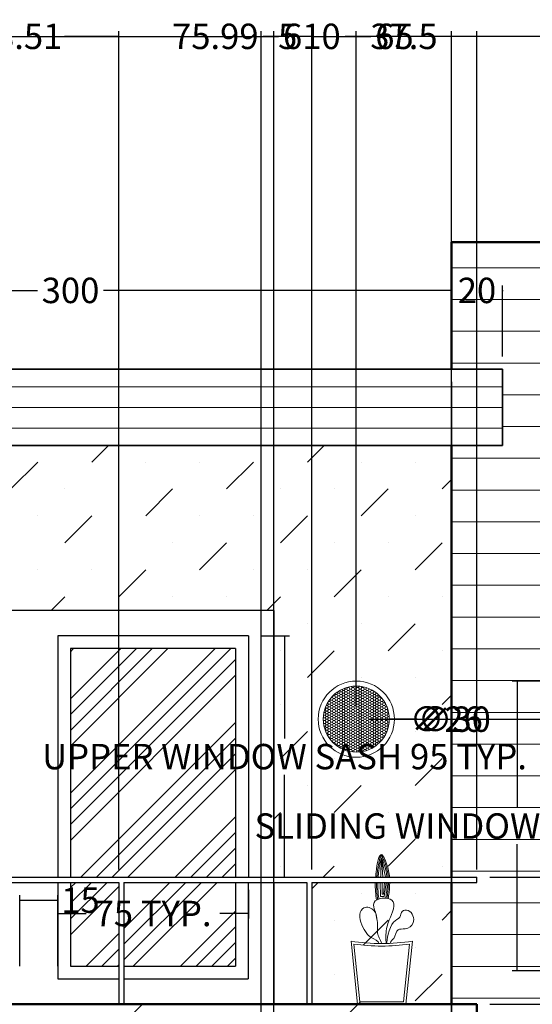
# Model space of a CAD drawing. Units: millimetres. Extents: x 301 to 1039, y -12 to 673.
# Tile 4 of 6: x 534 to 736, y 285 to 673. Entities that reach past the tile are written whole.
import ezdxf

# ---------------------------------------------------------------- set-up
doc = ezdxf.new("R2010")
doc.units = ezdxf.units.MM
doc.header["$MEASUREMENT"] = 0
for name, color, linetype, lineweight in [('A-ANNO-DIMS', 2, 'Continuous', 18), ('A-EQPM', 8, 'Continuous', 18), ('A-FLOR-HRAL', 6, 'Continuous', 25), ('A-GLAZ', 4, 'Continuous', 25), ('A-GLAZ-PATT', 8, 'Continuous', 13), ('A-ROOF', 1, 'Continuous', 35), ('A-WALL', 7, 'Continuous', 50), ('A-WALL-PATT', 9, 'Continuous', 13), ('L-PLNT', 3, 'Continuous', 18)]:
    doc.layers.add(name, color=color, linetype=linetype, lineweight=lineweight)
doc.styles.get("Standard").update_dxf_attribs({"font": 'arial.ttf'})
doc.dimstyles.get("Standard").update_dxf_attribs({"dimtxt": 10, "dimasz": 0.18, "dimexe": 2, "dimexo": 5, "dimgap": 2, "dimtad": 0, "dimtih": 1, "dimtoh": 1, "dimdec": 0, "dimzin": 0, "dimdsep": 46, "dimtxsty": 'Standard', "dimcen": 0.09, "dimadec": 0, "dimazin": 0, "dimtfac": 1, "dimtdec": 0, "dimtofl": 0, "dimtmove": 0, "dimatfit": 3, "dimfxl": 1, "dimtolj": 1, "dimtzin": 0, "dimarcsym": 0})

# ---------------------------------------------------------------- blocks, each defined once
blk = doc.blocks.new('WIN-SASH-UPPER')
for p, q in [((623.79, 430.09), (548.79, 430.09)), ((548.79, 430.09), (548.79, 400.52)), ((623.79, 430.09), (623.79, 400.52)), ((618.79, 425.09), (553.79, 425.09)), ((553.79, 425.09), (553.79, 400.52)), ((618.79, 425.09), (618.79, 400.52)), ((548.79, 400.52), (548.79, 335.09)), ((553.79, 400.52), (553.79, 335.09)), ((618.79, 400.52), (618.79, 335.09)), ((623.79, 400.52), (623.79, 335.09))]:
    blk.add_line(p, q)
blk = doc.blocks.new('*D12')
at = {"layer": 'A-ANNO-DIMS', "color": 0, "lineweight": -2, "transparency": 16777216}
for p, q in [((628.79, 430.09), (640.04, 430.09)), ((638.04, 429.91), (638.04, 389.76)), ((638.04, 335.27), (638.04, 375.41)), ((628.79, 335.09), (640.04, 335.09))]:
    blk.add_line(p, q, dxfattribs=at)
at = {"layer": 'A-ANNO-DIMS', "color": 0, "transparency": 16777216}
for points in [[(638.01, 429.91), (638.07, 429.91), (638.04, 430.09)], [(638.01, 335.27), (638.07, 335.27), (638.04, 335.09)]]:
    blk.add_solid(points, dxfattribs=at)
at = {"layer": 'Defpoints', "color": 0, "transparency": 16777216}
for p in [(623.79, 430.09), (638.04, 430.09), (623.79, 335.09)]:
    blk.add_point(p, dxfattribs=at)
at = {"layer": 'A-ANNO-DIMS', "color": 0, "transparency": 16777216, "insert": (638.04, 382.59), "char_height": 10, "attachment_point": 5}
blk.add_mtext('\\A1;UPPER WINDOW SASH 95 TYP.', dxfattribs=at)
blk = doc.blocks.new('*D13')
at = {"layer": 'A-ANNO-DIMS', "color": 0, "lineweight": -2, "transparency": 16777216}
for p, q in [((548.79, 330.09), (548.79, 318.84)), ((623.79, 330.09), (623.79, 318.84)), ((548.97, 320.84), (559.99, 320.84)), ((623.61, 320.84), (612.59, 320.84))]:
    blk.add_line(p, q, dxfattribs=at)
at = {"layer": 'A-ANNO-DIMS', "color": 0, "transparency": 16777216}
for points in [[(548.97, 320.87), (548.97, 320.81), (548.79, 320.84)], [(623.61, 320.87), (623.61, 320.81), (623.79, 320.84)]]:
    blk.add_solid(points, dxfattribs=at)
at = {"layer": 'Defpoints', "color": 0, "transparency": 16777216}
for p in [(548.79, 335.09), (623.79, 335.09), (623.79, 320.84)]:
    blk.add_point(p, dxfattribs=at)
at = {"layer": 'A-ANNO-DIMS', "color": 0, "transparency": 16777216, "insert": (586.29, 320.84), "char_height": 10, "attachment_point": 5}
blk.add_mtext('\\A1;75 TYP.', dxfattribs=at)
blk = doc.blocks.new('*D16')
at = {"layer": 'A-ANNO-DIMS', "color": 0, "lineweight": -2, "transparency": 16777216}
for p, q in [((741.69, 412.26), (727.59, 412.26)), ((729.59, 412.08), (729.59, 362.44)), ((729.59, 298.44), (729.59, 348.09)), ((741.69, 298.26), (727.59, 298.26))]:
    blk.add_line(p, q, dxfattribs=at)
at = {"layer": 'A-ANNO-DIMS', "color": 0, "transparency": 16777216}
for points in [[(729.56, 412.08), (729.62, 412.08), (729.59, 412.26)], [(729.56, 298.44), (729.62, 298.44), (729.59, 298.26)]]:
    blk.add_solid(points, dxfattribs=at)
at = {"layer": 'Defpoints', "color": 0, "transparency": 16777216}
for p in [(729.59, 412.26), (746.69, 412.26), (746.69, 298.26)]:
    blk.add_point(p, dxfattribs=at)
at = {"layer": 'A-ANNO-DIMS', "color": 0, "transparency": 16777216, "insert": (729.59, 355.26), "char_height": 10, "attachment_point": 5}
blk.add_mtext('\\A1;SLIDING WINDOW SASH 114 TYP.', dxfattribs=at)
blk = doc.blocks.new('*D20')
at = {"layer": 'A-ANNO-DIMS', "color": 0, "lineweight": -2, "transparency": 16777216}
for p, q in [((343.79, 30.09), (343.79, 668.09)), ((953.79, 30.09), (953.79, 668.09)), ((343.97, 666.09), (635.73, 666.09)), ((953.61, 666.09), (661.85, 666.09))]:
    blk.add_line(p, q, dxfattribs=at)
at = {"layer": 'A-ANNO-DIMS', "color": 0, "transparency": 16777216}
for points in [[(343.97, 666.12), (343.97, 666.06), (343.79, 666.09)], [(953.61, 666.12), (953.61, 666.06), (953.79, 666.09)]]:
    blk.add_solid(points, dxfattribs=at)
at = {"layer": 'Defpoints', "color": 0, "transparency": 16777216}
for p in [(953.79, 666.09), (343.79, 25.09), (953.79, 25.09)]:
    blk.add_point(p, dxfattribs=at)
at = {"layer": 'A-ANNO-DIMS', "color": 0, "transparency": 16777216, "insert": (648.79, 666.09), "char_height": 10, "attachment_point": 5}
blk.add_mtext('\\A1;610', dxfattribs=at)
blk = doc.blocks.new('*D26')
at = {"layer": 'A-ANNO-DIMS', "color": 0, "lineweight": -2, "transparency": 16777216}
for p, q in [((703.79, 530.09), (703.79, -7.91)), ((613.79, 30.09), (613.79, -7.91)), ((613.97, -5.91), (649.64, -5.91)), ((703.61, -5.91), (667.93, -5.91))]:
    blk.add_line(p, q, dxfattribs=at)
at = {"layer": 'A-ANNO-DIMS', "color": 0, "transparency": 16777216}
for points in [[(613.97, -5.88), (613.97, -5.94), (613.79, -5.91)], [(703.61, -5.88), (703.61, -5.94), (703.79, -5.91)]]:
    blk.add_solid(points, dxfattribs=at)
at = {"layer": 'Defpoints', "color": 0, "transparency": 16777216}
for p in [(703.79, 535.09), (613.79, 35.09), (703.79, -5.91)]:
    blk.add_point(p, dxfattribs=at)
at = {"layer": 'A-ANNO-DIMS', "color": 0, "transparency": 16777216, "insert": (658.79, -5.91), "char_height": 10, "attachment_point": 5}
blk.add_mtext('\\A1;90', dxfattribs=at)
blk = doc.blocks.new('*D27')
at = {"layer": 'A-ANNO-DIMS', "color": 0, "lineweight": -2, "transparency": 16777216}
for p, q in [((703.79, 530.09), (703.79, -7.91)), ((728.79, 155.09), (728.79, -7.91)), ((703.97, -5.91), (707, -5.91)), ((728.61, -5.91), (725.57, -5.91))]:
    blk.add_line(p, q, dxfattribs=at)
at = {"layer": 'A-ANNO-DIMS', "color": 0, "transparency": 16777216}
for points in [[(703.97, -5.88), (703.97, -5.94), (703.79, -5.91)], [(728.61, -5.88), (728.61, -5.94), (728.79, -5.91)]]:
    blk.add_solid(points, dxfattribs=at)
at = {"layer": 'Defpoints', "color": 0, "transparency": 16777216}
for p in [(703.79, 535.09), (728.79, 160.09), (728.79, -5.91)]:
    blk.add_point(p, dxfattribs=at)
at = {"layer": 'A-ANNO-DIMS', "color": 0, "transparency": 16777216, "insert": (716.29, -5.91), "char_height": 10, "attachment_point": 5}
blk.add_mtext('\\A1;25', dxfattribs=at)
blk = doc.blocks.new('*D44')
at = {"layer": 'A-ANNO-DIMS', "color": 0, "lineweight": -2, "transparency": 16777216}
for p, q in [((403.79, 540.09), (403.79, 568.09)), ((403.97, 566.09), (540.76, 566.09)), ((703.61, 566.09), (566.82, 566.09)), ((703.79, 540.09), (703.79, 568.09))]:
    blk.add_line(p, q, dxfattribs=at)
at = {"layer": 'A-ANNO-DIMS', "color": 0, "transparency": 16777216}
for points in [[(403.97, 566.12), (403.97, 566.06), (403.79, 566.09)], [(703.61, 566.12), (703.61, 566.06), (703.79, 566.09)]]:
    blk.add_solid(points, dxfattribs=at)
at = {"layer": 'Defpoints', "color": 0, "transparency": 16777216}
for p in [(703.79, 566.09), (403.79, 535.09), (703.79, 535.09)]:
    blk.add_point(p, dxfattribs=at)
at = {"layer": 'A-ANNO-DIMS', "color": 0, "transparency": 16777216, "insert": (553.79, 566.09), "char_height": 10, "attachment_point": 5}
blk.add_mtext('\\A1;300', dxfattribs=at)
blk = doc.blocks.new('*D45')
at = {"layer": 'A-ANNO-DIMS', "color": 0, "lineweight": -2, "transparency": 16777216}
for p, q in [((703.608413, 566.088152), (703.428413, 566.088152)), ((703.788413, 540.088152), (703.788413, 568.088152)), ((723.788413, 540.088152), (723.788413, 568.088152)), ((723.968413, 566.088152), (724.148413, 566.088152))]:
    blk.add_line(p, q, dxfattribs=at)
at = {"layer": 'A-ANNO-DIMS', "color": 0, "transparency": 16777216}
for points in [[(703.608413, 566.118152), (703.608413, 566.058152), (703.788413, 566.088152)], [(723.968413, 566.118152), (723.968413, 566.058152), (723.788413, 566.088152)]]:
    blk.add_solid(points, dxfattribs=at)
at = {"layer": 'Defpoints', "color": 0, "transparency": 16777216}
for p in [(723.788413, 566.088152), (703.788413, 535.088152), (723.788413, 535.088152)]:
    blk.add_point(p, dxfattribs=at)
at = {"layer": 'A-ANNO-DIMS', "color": 0, "transparency": 16777216, "insert": (713.788413, 566.088152), "char_height": 10, "attachment_point": 5}
blk.add_mtext('\\A1;20', dxfattribs=at)
blk = doc.blocks.new('*D52')
at = {"layer": 'A-ANNO-DIMS', "color": 0, "lineweight": -2, "transparency": 16777216}
for p, q in [((666.29, 402.33), (666.29, 668.09)), ((703.79, 265.09), (703.79, 668.09)), ((666.47, 666.09), (670.02, 666.09)), ((703.61, 666.09), (700.06, 666.09))]:
    blk.add_line(p, q, dxfattribs=at)
at = {"layer": 'A-ANNO-DIMS', "color": 0, "transparency": 16777216}
for points in [[(666.47, 666.12), (666.47, 666.06), (666.29, 666.09)], [(703.61, 666.12), (703.61, 666.06), (703.79, 666.09)]]:
    blk.add_solid(points, dxfattribs=at)
at = {"layer": 'Defpoints', "color": 0, "transparency": 16777216}
for p in [(703.79, 666.09), (666.29, 397.33), (703.79, 260.09)]:
    blk.add_point(p, dxfattribs=at)
at = {"layer": 'A-ANNO-DIMS', "color": 0, "transparency": 16777216, "insert": (685.04, 666.09), "char_height": 10, "attachment_point": 5}
blk.add_mtext('\\A1;37.5', dxfattribs=at)
blk = doc.blocks.new('*D56')
at = {"layer": 'A-ANNO-DIMS', "color": 0, "lineweight": -2, "transparency": 16777216}
for p, q in [((718.79, 335.09), (986.79, 335.09)), ((984.79, 334.91), (984.79, 317.19)), ((984.79, 285.27), (984.79, 302.98)), ((718.79, 285.09), (986.79, 285.09))]:
    blk.add_line(p, q, dxfattribs=at)
at = {"layer": 'A-ANNO-DIMS', "color": 0, "transparency": 16777216}
for points in [[(984.76, 334.91), (984.82, 334.91), (984.79, 335.09)], [(984.76, 285.27), (984.82, 285.27), (984.79, 285.09)]]:
    blk.add_solid(points, dxfattribs=at)
at = {"layer": 'Defpoints', "color": 0, "transparency": 16777216}
for p in [(713.79, 335.09), (984.79, 335.09), (713.79, 285.09)]:
    blk.add_point(p, dxfattribs=at)
at = {"layer": 'A-ANNO-DIMS', "color": 0, "transparency": 16777216, "insert": (984.79, 310.09), "char_height": 10, "attachment_point": 5}
blk.add_mtext('\\A1;50', dxfattribs=at)
blk = doc.blocks.new('*D57')
at = {"layer": 'A-ANNO-DIMS', "color": 0, "lineweight": -2, "transparency": 16777216}
for p, q in [((671.29, 397.33), (986.79, 397.33)), ((984.79, 397.15), (984.79, 373.32)), ((984.79, 335.27), (984.79, 359.11)), ((718.79, 335.09), (986.79, 335.09))]:
    blk.add_line(p, q, dxfattribs=at)
at = {"layer": 'A-ANNO-DIMS', "color": 0, "transparency": 16777216}
for points in [[(984.76, 397.15), (984.82, 397.15), (984.79, 397.33)], [(984.76, 335.27), (984.82, 335.27), (984.79, 335.09)]]:
    blk.add_solid(points, dxfattribs=at)
at = {"layer": 'Defpoints', "color": 0, "transparency": 16777216}
for p in [(666.29, 397.33), (984.79, 397.33), (713.79, 335.09)]:
    blk.add_point(p, dxfattribs=at)
at = {"layer": 'A-ANNO-DIMS', "color": 0, "transparency": 16777216, "insert": (984.79, 366.21), "char_height": 10, "attachment_point": 5}
blk.add_mtext('\\A1;62.25', dxfattribs=at)
blk = doc.blocks.new('*D60')
at = {"layer": 'A-ANNO-DIMS', "color": 0, "lineweight": -2, "transparency": 16777216}
for p, q in [((494.29, 338.09), (494.29, 668.09)), ((572.8, 338.09), (572.8, 668.09)), ((494.47, 666.09), (515.68, 666.09)), ((572.62, 666.09), (551.41, 666.09))]:
    blk.add_line(p, q, dxfattribs=at)
at = {"layer": 'A-ANNO-DIMS', "color": 0, "transparency": 16777216}
for points in [[(494.47, 666.12), (494.47, 666.06), (494.29, 666.09)], [(572.62, 666.12), (572.62, 666.06), (572.8, 666.09)]]:
    blk.add_solid(points, dxfattribs=at)
at = {"layer": 'Defpoints', "color": 0, "transparency": 16777216}
for p in [(572.8, 666.09), (494.29, 333.09), (572.8, 333.09)]:
    blk.add_point(p, dxfattribs=at)
at = {"layer": 'A-ANNO-DIMS', "color": 0, "transparency": 16777216, "insert": (533.54, 666.09), "char_height": 10, "attachment_point": 5}
blk.add_mtext('\\A1;78.51', dxfattribs=at)
blk = doc.blocks.new('*D61')
at = {"layer": 'A-ANNO-DIMS', "color": 0, "lineweight": -2, "transparency": 16777216}
for p, q in [((572.8, 338.09), (572.8, 668.09)), ((648.79, 338.09), (648.79, 668.09)), ((572.98, 666.09), (591.95, 666.09)), ((648.61, 666.09), (629.64, 666.09))]:
    blk.add_line(p, q, dxfattribs=at)
at = {"layer": 'A-ANNO-DIMS', "color": 0, "transparency": 16777216}
for points in [[(572.98, 666.12), (572.98, 666.06), (572.8, 666.09)], [(648.61, 666.12), (648.61, 666.06), (648.79, 666.09)]]:
    blk.add_solid(points, dxfattribs=at)
at = {"layer": 'Defpoints', "color": 0, "transparency": 16777216}
for p in [(648.79, 666.09), (572.8, 333.09), (648.79, 333.09)]:
    blk.add_point(p, dxfattribs=at)
at = {"layer": 'A-ANNO-DIMS', "color": 0, "transparency": 16777216, "insert": (610.79, 666.09), "char_height": 10, "attachment_point": 5}
blk.add_mtext('\\A1;75.99', dxfattribs=at)
blk = doc.blocks.new('*D62')
at = {"layer": 'A-ANNO-DIMS', "color": 0, "lineweight": -2, "transparency": 16777216}
for p, q in [((648.79, 338.09), (648.79, 668.09)), ((713.79, 338.09), (713.79, 668.09)), ((648.97, 666.09), (672.06, 666.09)), ((713.61, 666.09), (690.52, 666.09))]:
    blk.add_line(p, q, dxfattribs=at)
at = {"layer": 'A-ANNO-DIMS', "color": 0, "transparency": 16777216}
for points in [[(648.97, 666.12), (648.97, 666.06), (648.79, 666.09)], [(713.61, 666.12), (713.61, 666.06), (713.79, 666.09)]]:
    blk.add_solid(points, dxfattribs=at)
at = {"layer": 'Defpoints', "color": 0, "transparency": 16777216}
for p in [(713.79, 666.09), (648.79, 333.09), (713.79, 333.09)]:
    blk.add_point(p, dxfattribs=at)
at = {"layer": 'A-ANNO-DIMS', "color": 0, "transparency": 16777216, "insert": (681.29, 666.09), "char_height": 10, "attachment_point": 5}
blk.add_mtext('\\A1;65', dxfattribs=at)
blk = doc.blocks.new('*D63')
at = {"layer": 'A-ANNO-DIMS', "color": 0, "lineweight": -2, "transparency": 16777216}
for p, q in [((533.79, 300.09), (533.79, 328.09)), ((533.97, 326.09), (548.61, 326.09)), ((548.79, 300.09), (548.79, 328.09)), ((548.79, 326.09), (548.97, 326.09))]:
    blk.add_line(p, q, dxfattribs=at)
at = {"layer": 'A-ANNO-DIMS', "color": 0, "transparency": 16777216}
for points in [[(533.97, 326.12), (533.97, 326.06), (533.79, 326.09)], [(548.61, 326.12), (548.61, 326.06), (548.79, 326.09)]]:
    blk.add_solid(points, dxfattribs=at)
at = {"layer": 'Defpoints', "color": 0, "transparency": 16777216}
for p in [(548.79, 326.09), (533.79, 295.09), (548.79, 295.09)]:
    blk.add_point(p, dxfattribs=at)
at = {"layer": 'A-ANNO-DIMS', "color": 0, "transparency": 16777216, "insert": (557.7, 326.09), "char_height": 10, "attachment_point": 5}
blk.add_mtext('\\A1;15', dxfattribs=at)
blk = doc.blocks.new('*D72')
at = {"layer": 'A-ANNO-DIMS', "color": 0, "lineweight": -2, "transparency": 16777216}
for p, q in [((628.79, 190.09), (628.79, 668.09)), ((633.79, 185.09), (633.79, 668.09)), ((628.97, 666.09), (633.61, 666.09)), ((633.79, 666.09), (633.97, 666.09))]:
    blk.add_line(p, q, dxfattribs=at)
at = {"layer": 'A-ANNO-DIMS', "color": 0, "transparency": 16777216}
for points in [[(628.97, 666.12), (628.97, 666.06), (628.79, 666.09)], [(633.61, 666.12), (633.61, 666.06), (633.79, 666.09)]]:
    blk.add_solid(points, dxfattribs=at)
at = {"layer": 'Defpoints', "color": 0, "transparency": 16777216}
for p in [(633.79, 666.09), (628.79, 185.09), (633.79, 180.09)]:
    blk.add_point(p, dxfattribs=at)
at = {"layer": 'A-ANNO-DIMS', "color": 0, "transparency": 16777216, "insert": (639.28, 666.09), "char_height": 10, "attachment_point": 5}
blk.add_mtext('\\A1;5', dxfattribs=at)
blk = doc.blocks.new('*D79')
at = {"layer": 'A-ANNO-DIMS', "color": 0, "lineweight": -2, "transparency": 16777216}
for p, q in [((666.2, 397.33), (666.38, 397.33)), ((666.29, 397.24), (666.29, 397.42)), ((690.29, 397.33), (681.47, 397.33))]:
    blk.add_line(p, q, dxfattribs=at)
at = {"layer": 'A-ANNO-DIMS', "color": 0, "transparency": 16777216}
blk.add_solid([(681.47, 397.36), (681.47, 397.3), (681.29, 397.33)], dxfattribs=at)
at = {"layer": 'Defpoints', "color": 0, "transparency": 16777216}
for p in [(651.29, 397.34), (681.29, 397.33)]:
    blk.add_point(p, dxfattribs=at)
at = {"layer": 'A-ANNO-DIMS', "color": 0, "transparency": 16777216, "insert": (704.88, 397.33), "char_height": 10, "attachment_point": 5}
blk.add_mtext('\\A1;∅30', dxfattribs=at)
blk = doc.blocks.new('*D80')
at = {"layer": 'A-ANNO-DIMS', "color": 0, "lineweight": -2, "transparency": 16777216}
for p, q in [((666.2, 397.33), (666.38, 397.33)), ((666.29, 397.24), (666.29, 397.42)), ((687.09, 397.33), (679.47, 397.33))]:
    blk.add_line(p, q, dxfattribs=at)
at = {"layer": 'A-ANNO-DIMS', "color": 0, "transparency": 16777216}
blk.add_solid([(679.47, 397.36), (679.47, 397.3), (679.29, 397.33)], dxfattribs=at)
at = {"layer": 'Defpoints', "color": 0, "transparency": 16777216}
for p in [(653.29, 397.34), (679.29, 397.33)]:
    blk.add_point(p, dxfattribs=at)
at = {"layer": 'A-ANNO-DIMS', "color": 0, "transparency": 16777216, "insert": (701.69, 397.33), "char_height": 10, "attachment_point": 5}
blk.add_mtext('\\A1;∅26', dxfattribs=at)

msp = doc.modelspace()

# ---------------------------------------------------------------- hatches: boundary and pattern name
at = {"layer": 'A-EQPM'}
h = msp.add_hatch(dxfattribs=at)
h.set_pattern_fill('HONEY', color=256, scale=5)
h.paths.add_polyline_path([(653.292, 397.334, 1), (679.292, 397.334, 1)])
at = {"layer": 'A-GLAZ-PATT'}
h = msp.add_hatch(dxfattribs=at)
h.set_pattern_fill('ANSI34', color=256, scale=35)
h.paths.add_polyline_path([(528.788, 400.52), (528.788, 425.088), (463.788, 425.088), (463.788, 400.52), (463.788, 335.088), (528.788, 335.088)])
h.paths.add_polyline_path([(494.288, 333.088), (463.788, 333.088), (463.788, 300.088), (494.288, 300.088)])
h.paths.add_polyline_path([(528.788, 333.088), (496.288, 333.088), (496.288, 300.088), (528.788, 300.088)])
h.paths.add_polyline_path([(618.788, 400.52), (618.788, 425.088), (553.788, 425.088), (553.788, 400.52), (553.788, 335.088), (618.788, 335.088)])
h.paths.add_polyline_path([(618.788, 333.088), (574.798, 333.088), (574.798, 300.088), (618.788, 300.088)])
h.paths.add_polyline_path([(572.798, 333.088), (553.788, 333.088), (553.788, 300.088), (572.798, 300.088)])
h.paths.add_polyline_path([(501.288, 180.088), (433.788, 180.088), (433.788, 110.088), (501.288, 110.088)])
h.paths.add_polyline_path([(573.788, 180.088), (506.288, 180.088), (506.288, 110.088), (573.788, 110.088)])
h.paths.add_polyline_path([(573.788, 210.088), (506.288, 210.088), (506.288, 185.088), (573.788, 185.088)])
h.paths.add_polyline_path([(501.288, 210.088), (433.788, 210.088), (433.788, 185.088), (501.288, 185.088)])
h.paths.add_polyline_path([(797.687, 412.264), (746.687, 412.264), (746.687, 298.264), (797.687, 298.264)])
h.paths.add_polyline_path([(860.687, 412.264), (809.687, 412.264), (809.687, 298.264), (860.687, 298.264)])
at = {"layer": 'A-WALL-PATT'}
h = msp.add_hatch(dxfattribs=at)
h.set_pattern_fill('ANSI31', color=256, scale=100, angle=135)
h.paths.add_polyline_path([(903.788, 585.088), (703.788, 585.088), (703.788, 535.088), (723.788, 535.088), (723.788, 505.088), (703.788, 505.088), (703.788, 335.088), (713.788, 335.088), (713.788, 333.088), (703.788, 333.088), (703.788, 285.088), (713.788, 285.088), (713.788, 265.672), (903.788, 265.672)])
h.paths.add_polyline_path([(868.687, 420.264), (868.687, 290.264), (738.687, 290.264), (738.687, 420.264)], flags=16)
h.paths.add_polyline_path([(866.687, 418.264), (866.687, 292.264), (740.687, 292.264), (740.687, 418.264)], flags=0)
h.paths.add_polyline_path([(861.687, 413.264), (861.687, 297.264), (745.687, 297.264), (745.687, 413.264)], flags=0)
h.paths.add_polyline_path([(860.687, 412.264), (860.687, 298.264), (809.687, 298.264), (809.687, 412.264)], flags=0)
h.paths.add_polyline_path([(797.687, 412.264), (797.687, 298.264), (746.687, 298.264), (746.687, 412.264)], flags=0)
h = msp.add_hatch(dxfattribs=at)
h.set_pattern_fill('ANSI31', color=256, scale=65, angle=135)
h.paths.add_polyline_path([(723.788, 535.088), (703.788, 535.088), (403.788, 535.088), (393.788, 535.088), (393.788, 505.088), (403.788, 505.088), (703.788, 505.088), (723.788, 505.088)])
h = msp.add_hatch(dxfattribs=at)
h.set_pattern_fill('MUDST', color=256, scale=60, angle=45)
edge = h.paths.add_edge_path()
edge.add_line((703.788, 505.088), (403.788, 505.088))
edge.add_line((403.788, 505.088), (403.788, 335.088))
edge.add_line((403.788, 335.088), (448.788, 335.088))
edge.add_line((448.788, 335.088), (448.788, 400.52))
edge.add_line((448.788, 400.52), (448.788, 440.088))
edge.add_line((448.788, 440.088), (633.788, 440.088))
edge.add_line((633.788, 440.088), (633.788, 400.52))
edge.add_line((633.788, 400.52), (633.788, 335.088))
edge.add_line((633.788, 335.088), (673.88, 335.088))
edge.add_spline(control_points=[(673.88, 335.088), (673.929, 335.734), (674.283, 339.462), (675.587, 346.794), (678.602, 339.909), (679.226, 336.718), (679.369, 335.088)], knot_values=[26.7052686, 26.7052686, 26.7052686, 26.7052686, 28.3156814, 35.5227919, 39.6456178, 44.5318346, 44.5318346, 44.5318346, 44.5318346], degree=3, periodic=0)
edge.add_line((679.369, 335.088), (703.788, 335.088))
edge.add_line((703.788, 335.088), (703.788, 505.088))
h.paths.add_polyline_path([(681.292, 397.334, -1), (651.292, 397.334, -1)], flags=16)
h.paths.add_polyline_path([(679.292, 397.334, -1), (653.292, 397.334, -1)], flags=0)
h.paths.add_polyline_path([(448.788, 333.088), (403.788, 333.088), (403.788, 285.088), (448.788, 285.088)])
h.paths.add_polyline_path([(613.788, 260.088), (713.788, 260.088), (713.788, 285.088), (403.788, 285.088), (393.788, 285.088), (393.788, 35.088), (403.788, 35.088), (613.788, 35.088)])
h.paths.add_polyline_path([(578.788, 215.088), (578.788, 105.088), (428.788, 105.088), (428.788, 215.088)], flags=16)
h.paths.add_polyline_path([(501.288, 210.088), (501.288, 185.088), (433.788, 185.088), (433.788, 210.088)], flags=0)
h.paths.add_polyline_path([(501.288, 180.088), (501.288, 110.088), (433.788, 110.088), (433.788, 180.088)], flags=0)
h.paths.add_polyline_path([(506.288, 210.088), (573.788, 210.088), (573.788, 185.088), (506.288, 185.088)], flags=0)
h.paths.add_polyline_path([(506.288, 180.088), (573.788, 180.088), (573.788, 110.088), (506.288, 110.088)], flags=0)
edge = h.paths.add_edge_path()
edge.add_spline(control_points=[(675.148, 309.006), (675.282, 309.92), (671.965, 311.304), (670.019, 313.17), (668.379, 316.485), (667.076, 320.028), (669.149, 324.142), (672.687, 322.877), (673.644, 321.553), (673.786, 321.296)], knot_values=[12.4980994, 12.4980994, 12.4980994, 12.4980994, 15.7345293, 18.1242776, 22.0598536, 26.1694355, 29.2709867, 33.3603853, 34.273637, 34.273637, 34.273637, 34.273637], degree=3, periodic=0)
edge.add_spline(control_points=[(673.786, 321.296), (673.373, 322.666), (672.565, 324.662), (673.805, 325.84), (674.246, 326.099)], knot_values=[12.3304253, 12.3304253, 12.3304253, 12.3304253, 16.1943692, 17.6683934, 17.6683934, 17.6683934, 17.6683934], degree=3, periodic=0)
edge.add_spline(control_points=[(674.246, 326.099), (673.92, 328.298), (673.697, 330.39), (673.774, 333.088)], knot_values=[46.2924512, 46.2924512, 46.2924512, 46.2924512, 53.8278009, 53.8278009, 53.8278009, 53.8278009], degree=3, periodic=0)
edge.add_line((673.774, 333.088), (648.788, 333.088))
edge.add_line((648.788, 333.088), (648.788, 285.088))
edge.add_line((648.788, 285.088), (666.788, 285.088))
edge.add_line((666.788, 285.088), (664.215, 309.96))
edge.add_arc((676.288, 385.148), 76.15, 260.87778, 269.14183)
edge = h.paths.add_edge_path()
edge.add_line((703.788, 333.088), (679.453, 333.088))
edge.add_spline(control_points=[(679.453, 333.088), (679.452, 331.277), (679.21, 329.205), (678.936, 327.067), (678.889, 326.706)], knot_values=[17.8386285, 17.8386285, 17.8386285, 17.8386285, 23.5111371, 24.6594022, 24.6594022, 24.6594022, 24.6594022], degree=3, periodic=0)
edge.add_spline(control_points=[(678.889, 326.706), (678.729, 326.741), (678.565, 326.771), (678.396, 326.794)], knot_values=[21.2892091, 21.2892091, 21.2892091, 21.2892091, 21.7264211, 21.7264211, 21.7264211, 21.7264211], degree=3, periodic=0)
edge.add_spline(control_points=[(678.396, 326.794), (678.233, 326.816), (678.067, 326.832), (677.898, 326.842)], knot_values=[20.8675669, 20.8675669, 20.8675669, 20.8675669, 21.2892091, 21.2892091, 21.2892091, 21.2892091], degree=3, periodic=0)
edge.add_spline(control_points=[(677.898, 326.842), (676.995, 326.898), (676.024, 326.786), (675.195, 326.517)], knot_values=[18.611077, 18.611077, 18.611077, 18.611077, 20.8675669, 20.8675669, 20.8675669, 20.8675669], degree=3, periodic=0)
edge.add_spline(control_points=[(675.195, 326.517), (675.029, 326.464), (674.869, 326.404), (674.716, 326.337)], knot_values=[18.1593829, 18.1593829, 18.1593829, 18.1593829, 18.611077, 18.611077, 18.611077, 18.611077], degree=3, periodic=0)
edge.add_spline(control_points=[(674.716, 326.337), (674.55, 326.265), (674.392, 326.186), (674.246, 326.099)], knot_values=[17.6683934, 17.6683934, 17.6683934, 17.6683934, 18.1593829, 18.1593829, 18.1593829, 18.1593829], degree=3, periodic=0)
edge.add_spline(control_points=[(674.246, 326.099), (673.805, 325.84), (672.565, 324.662), (673.373, 322.666), (673.786, 321.296)], knot_values=[12.3304253, 12.3304253, 12.3304253, 12.3304253, 13.8044495, 17.6683934, 17.6683934, 17.6683934, 17.6683934], degree=3, periodic=0)
edge.add_spline(control_points=[(673.786, 321.296), (674.162, 320.613), (674.301, 319.823), (674.341, 318.987)], knot_values=[10.0649388, 10.0649388, 10.0649388, 10.0649388, 12.4980994, 12.4980994, 12.4980994, 12.4980994], degree=3, periodic=0)
edge.add_spline(control_points=[(674.341, 318.987), (674.206, 319.737), (674.024, 320.504), (673.786, 321.296)], knot_values=[10.094462, 10.094462, 10.094462, 10.094462, 12.3304253, 12.3304253, 12.3304253, 12.3304253], degree=3, periodic=0)
edge.add_spline(control_points=[(673.786, 321.296), (673.644, 321.553), (672.687, 322.877), (669.149, 324.142), (667.076, 320.028), (668.379, 316.485), (670.019, 313.17), (671.965, 311.304), (675.282, 309.92), (675.148, 309.006)], knot_values=[12.4980994, 12.4980994, 12.4980994, 12.4980994, 13.4113511, 17.5007497, 20.6023009, 24.7118828, 28.6474588, 31.0372071, 34.273637, 34.273637, 34.273637, 34.273637], degree=3, periodic=0)
edge.add_arc((676.288, 385.148), 76.15, 260.87778, 269.14183, ccw=False)
edge.add_line((664.215, 309.96), (666.788, 285.088))
edge.add_line((666.788, 285.088), (703.788, 285.088))
edge.add_line((703.788, 285.088), (703.788, 333.088))
h.paths.add_polyline_path([(687.234, 308.777), (684.887, 286.088), (667.69, 286.088), (665.343, 308.777, 0.0712952)], flags=16)
h.paths.add_polyline_path([(903.788, 265.672), (713.788, 265.672), (713.788, 260.088), (703.788, 260.088), (703.788, 35.088), (728.788, 35.088), (728.788, 160.088), (878.788, 160.088), (878.788, 35.088), (903.788, 35.088)])

# ---------------------------------------------------------------- linework, layer by layer
at = {"layer": 'A-EQPM'}
for radius in [15, 13]:
    msp.add_circle((666.292, 397.334), radius, dxfattribs=at)
at = {"layer": 'A-FLOR-HRAL'}
for p, q in [((396.788, 335.088), (713.788, 335.088)), ((713.788, 333.088), (713.788, 335.088)), ((496.288, 333.088), (572.798, 333.088)), ((572.798, 333.088), (572.798, 285.088)), ((574.798, 333.088), (574.798, 285.088)), ((574.798, 333.088), (646.788, 333.088)), ((646.788, 333.088), (646.788, 285.088)), ((648.788, 333.088), (648.788, 285.088)), ((648.788, 333.088), (713.788, 333.088))]:
    msp.add_line(p, q, dxfattribs=at)
at = {"layer": 'A-GLAZ'}
for p, q in [((633.788, 440.088), (448.788, 440.088)), ((633.788, 440.088), (633.788, 400.52)), ((633.788, 400.52), (633.788, 335.088)), ((548.788, 333.088), (548.788, 295.088)), ((553.788, 333.088), (553.788, 300.088)), ((618.788, 333.088), (618.788, 300.088)), ((623.788, 333.088), (623.788, 295.088)), ((633.788, 333.088), (633.788, 285.088)), ((553.788, 300.088), (572.798, 300.088)), ((574.798, 300.088), (618.788, 300.088)), ((548.788, 295.088), (572.798, 295.088)), ((574.798, 295.088), (623.788, 295.088))]:
    msp.add_line(p, q, dxfattribs=at)
at = {"layer": 'A-ROOF'}
for p, q in [((703.788, 535.088), (403.788, 535.088)), ((703.788, 535.088), (723.788, 535.088)), ((723.788, 535.088), (723.788, 505.088)), ((703.788, 505.088), (403.788, 505.088)), ((723.788, 505.088), (703.788, 505.088))]:
    msp.add_line(p, q, dxfattribs=at)
at = {"layer": 'A-WALL'}
for p, q in [((903.788, 585.088), (703.788, 585.088)), ((703.788, 585.088), (703.788, 535.088)), ((703.788, 505.088), (703.788, 335.088)), ((703.788, 333.088), (703.788, 285.088)), ((403.788, 285.088), (713.788, 285.088)), ((703.788, 285.088), (713.788, 285.088)), ((713.788, 260.088), (713.788, 285.088))]:
    msp.add_line(p, q, dxfattribs=at)
at = {"layer": 'L-PLNT'}
for p, q in [((676.18, 342.654), (676.785, 335.088)), ((676.18, 342.654), (677.802, 335.088)), ((675.653, 333.088), (675.848, 327.548)), ((676.466, 333.088), (676.42, 328.439)), ((677.016, 328.433), (677.427, 333.088)), ((677.286, 327.578), (678.048, 333.088)), ((675.848, 327.548), (677.286, 327.578)), ((676.42, 328.439), (677.016, 328.433)), ((664.215, 309.96), (666.788, 285.088)), ((665.343, 308.777), (667.69, 286.088)), ((687.234, 308.777), (684.887, 286.088)), ((688.361, 309.96), (685.788, 285.088)), ((667.69, 286.088), (684.887, 286.088))]:
    msp.add_line(p, q, dxfattribs=at)
for radius, start, end in [(76.15, 260.87778, 279.12222), (77.15, 261.84397, 278.15603)]:
    msp.add_arc((676.288, 385.148), radius, start, end, dxfattribs=at)
for points, knots in [([(679.369, 335.088), (679.226, 336.718), (678.602, 339.909), (675.587, 346.794), (674.283, 339.462), (673.929, 335.734), (673.88, 335.088)], [26.7052686, 26.7052686, 26.7052686, 26.7052686, 31.5914854, 35.7143113, 42.9214218, 44.5318346, 44.5318346, 44.5318346, 44.5318346]), ([(676.1, 343.708), (676.01, 343.507), (675.92, 343.306), (675.83, 343.105), (675.792, 343.02), (675.755, 342.935), (675.717, 342.843), (675.636, 342.645), (675.556, 342.413), (675.402, 341.897), (675.328, 341.614), (675.059, 340.465), (674.889, 339.474), (674.671, 337.918), (674.602, 337.35), (674.476, 336.205), (674.423, 335.633), (674.381, 335.088)], [37.061146, 37.061146, 37.061146, 37.061146, 37.8954901, 37.8954901, 37.8954901, 38.2481688, 38.2481688, 38.2481688, 39.0063302, 39.0063302, 39.7644915, 39.7644915, 41.893887, 41.893887, 43.1281752, 43.1281752, 44.4997243, 44.4997243, 44.4997243, 44.4997243]), ([(676.18, 342.654), (676.122, 342.513), (676.062, 342.347), (675.856, 341.694), (675.713, 341.106), (675.459, 339.824), (675.346, 339.128), (675.155, 337.769), (675.076, 337.108), (674.96, 336.001), (674.917, 335.535), (674.883, 335.088)], [38.2481688, 38.2481688, 38.2481688, 38.2481688, 38.8481154, 38.8481154, 40.3660708, 40.3660708, 41.8840262, 41.8840262, 43.3333987, 43.3333987, 44.4678483, 44.4678483, 44.4678483, 44.4678483]), ([(676.18, 342.654), (676.079, 340.533), (675.955, 337.915), (675.884, 335.549), (675.858, 335.088)], [0, 0, 0, 0, 6.2000341, 7.6585671, 7.6585671, 7.6585671, 7.6585671]), ([(678.867, 335.088), (678.819, 335.619), (678.75, 336.16), (678.577, 337.182), (678.48, 337.658), (678.257, 338.586), (678.135, 339.036), (677.883, 339.862), (677.76, 340.235), (677.492, 340.986), (677.348, 341.36), (677.004, 342.169), (676.802, 342.587), (676.609, 342.91), (676.554, 343.001), (676.501, 343.085), (676.447, 343.168), (676.394, 343.25), (676.341, 343.333), (676.288, 343.415), (676.226, 343.512), (676.163, 343.61), (676.1, 343.708)], [26.7501024, 26.7501024, 26.7501024, 26.7501024, 28.3769713, 28.3769713, 29.7407193, 29.7407193, 30.9711156, 30.9711156, 31.940783, 31.940783, 32.9104504, 32.9104504, 34.1777477, 34.1777477, 34.1777477, 34.5351296, 34.5351296, 34.5351296, 34.8872675, 34.8872675, 34.8872675, 35.3057376, 35.3057376, 35.3057376, 35.3057376]), ([(678.365, 335.088), (678.323, 335.543), (678.265, 336.006), (678.116, 336.926), (678.027, 337.381), (677.815, 338.299), (677.693, 338.76), (677.45, 339.572), (677.338, 339.918), (677.094, 340.619), (676.962, 340.971), (676.649, 341.739), (676.464, 342.142), (676.252, 342.529), (676.215, 342.594), (676.18, 342.654)], [26.796786, 26.796786, 26.796786, 26.796786, 28.2234795, 28.2234795, 29.5686137, 29.5686137, 30.8636353, 30.8636353, 31.7881294, 31.7881294, 32.7126235, 32.7126235, 33.9185564, 33.9185564, 34.1777477, 34.1777477, 34.1777477, 34.1777477]), ([(674.274, 333.088), (674.256, 332.456), (674.254, 331.859), (674.301, 329.702), (674.442, 328.306), (674.663, 326.704), (674.689, 326.521), (674.716, 326.337)], [46.2789934, 46.2789934, 46.2789934, 46.2789934, 48.0653283, 48.0653283, 53.0024814, 53.0024814, 53.6380427, 53.6380427, 53.6380427, 53.6380427]), ([(674.774, 333.088), (674.76, 332.593), (674.756, 332.12), (674.777, 330.14), (674.894, 328.803), (675.106, 327.146), (675.15, 326.833), (675.195, 326.517)], [46.2651407, 46.2651407, 46.2651407, 46.2651407, 47.681516, 47.681516, 52.4123893, 52.4123893, 53.5130856, 53.5130856, 53.5130856, 53.5130856]), ([(677.898, 326.842), (677.97, 327.394), (678.04, 327.941), (678.214, 329.361), (678.311, 330.222), (678.423, 331.748), (678.453, 332.413), (678.453, 333.088)], [17.8461463, 17.8461463, 17.8461463, 17.8461463, 19.6027525, 19.6027525, 22.4555385, 22.4555385, 24.6589166, 24.6589166, 24.6589166, 24.6589166]), ([(678.396, 326.794), (678.464, 327.313), (678.529, 327.828), (678.761, 329.708), (678.906, 331.048), (678.95, 332.643), (678.953, 332.865), (678.953, 333.088)], [17.8630139, 17.8630139, 17.8630139, 17.8630139, 19.5132079, 19.5132079, 23.9450896, 23.9450896, 24.6594628, 24.6594628, 24.6594628, 24.6594628]), ([(678.889, 326.706), (678.936, 327.067), (679.21, 329.205), (679.452, 331.277), (679.453, 333.088)], [17.8386285, 17.8386285, 17.8386285, 17.8386285, 18.9868936, 24.6594022, 24.6594022, 24.6594022, 24.6594022]), ([(674.65, 313.139), (674.763, 315.826), (674.614, 319.598), (671.712, 326.77), (683.707, 327.873), (678.999, 318.174), (677.831, 313.975), (677.979, 309.446), (678.055, 309.018)], [4.1270645, 4.1270645, 4.1270645, 4.1270645, 12.3304253, 16.1943692, 23.3050104, 31.1479744, 37.1348905, 40.5679872, 40.5679872, 40.5679872, 40.5679872]), ([(674.341, 318.987), (674.286, 320.137), (673.749, 322.497), (669.149, 324.142), (667.076, 320.028), (668.379, 316.485), (670.019, 313.17), (671.965, 311.304), (675.282, 309.92), (675.148, 309.006)], [10.0649388, 10.0649388, 10.0649388, 10.0649388, 13.4113511, 17.5007497, 20.6023009, 24.7118828, 28.6474588, 31.0372071, 34.273637, 34.273637, 34.273637, 34.273637]), ([(678.157, 309.02), (678.395, 309.894), (679.168, 317.621), (683.755, 318.771), (683.83, 322.136), (688.144, 322.466), (689.921, 316.937), (686.023, 314.397), (681.869, 315.107), (681.802, 311.097), (679.66, 309.848), (679.634, 309.071)], [41.8776927, 41.8776927, 41.8776927, 41.8776927, 49.4421427, 52.6297816, 55.0619385, 57.4321504, 62.7221473, 66.6479611, 69.439093, 73.2426653, 75.6423686, 75.6423686, 75.6423686, 75.6423686])]:
    msp.add_open_spline(points, degree=3, knots=knots, dxfattribs=at)
for points in [[(673.774, 333.088), (673.697, 330.39), (673.92, 328.298), (674.246, 326.099)], [(676.39, 308.997), (675.524, 310.638), (674.986, 311.85), (674.65, 313.139)], [(677.288, 308.004), (677.288, 308), (677.288, 307.997), (677.288, 307.993)]]:
    msp.add_open_spline(points, degree=3, dxfattribs=at)

# ---------------------------------------------------------------- block references
at = {"layer": 'A-GLAZ'}
msp.add_blockref('WIN-SASH-UPPER', (0, 0), dxfattribs=at)

# ---------------------------------------------------------------- dimensions: what is measured, and where the dimension line sits
at = {"layer": 'A-ANNO-DIMS'}
for base, p1, p2, override, picture, middle in [((953.788, 666.088), (343.788, 25.088), (953.788, 25.088), {"dimdec": 0, "dimlfac": 1, "dimrnd": 0, "dimzin": 0, "dimdsep": 46, "dimlunit": 2}, '*D20', (648.788, 666.088)), ((572.798, 666.088), (494.288, 333.088), (572.798, 333.088), {"dimdec": 2, "dimlfac": 1, "dimrnd": 0, "dimzin": 0, "dimdsep": 46, "dimlunit": 2}, '*D60', (533.543, 666.088)), ((648.788, 666.088), (572.798, 333.088), (648.788, 333.088), {"dimdec": 2, "dimlfac": 1, "dimrnd": 0, "dimzin": 0, "dimdsep": 46, "dimlunit": 2}, '*D61', (610.793, 666.088)), ((633.788, 666.088), (628.788, 185.088), (633.788, 180.088), {"dimdec": 0, "dimlfac": 1, "dimrnd": 0, "dimzin": 0, "dimdsep": 46, "dimlunit": 2}, '*D72', (639.284, 666.088)), ((713.788, 666.088), (648.788, 333.088), (713.788, 333.088), {"dimdec": 0, "dimlfac": 1, "dimrnd": 0, "dimzin": 0, "dimdsep": 46, "dimlunit": 2}, '*D62', (681.288, 666.088)), ((703.788, 666.088), (666.292, 397.334), (703.788, 260.088), {"dimdec": 1, "dimlfac": 1, "dimrnd": 0, "dimzin": 0, "dimdsep": 46, "dimlunit": 2}, '*D52', (685.04, 666.088)), ((703.788, 566.088), (403.788, 535.088), (703.788, 535.088), {"dimdec": 0, "dimlfac": 1, "dimrnd": 0, "dimzin": 0, "dimdsep": 46, "dimlunit": 2}, '*D44', (553.788, 566.088)), ((723.788, 566.088), (703.788, 535.088), (723.788, 535.088), {"dimdec": 0, "dimlfac": 1, "dimrnd": 0, "dimzin": 0, "dimdsep": 46, "dimlunit": 2}, '*D45', (713.788, 566.088)), ((703.788, -5.912), (613.788, 35.088), (703.788, 535.088), {"dimdec": 0, "dimlfac": 1, "dimrnd": 0, "dimzin": 0, "dimdsep": 46, "dimlunit": 2}, '*D26', (658.788, -5.912)), ((728.788, -5.912), (703.788, 535.088), (728.788, 160.088), {"dimdec": 0, "dimlfac": 1, "dimrnd": 0, "dimzin": 0, "dimdsep": 46, "dimlunit": 2}, '*D27', (716.288, -5.912)), ((548.788, 326.088), (533.788, 295.088), (548.788, 295.088), {"dimdec": 0, "dimlfac": 1, "dimrnd": 0, "dimzin": 0, "dimdsep": 46, "dimlunit": 2}, '*D63', (557.698, 326.088))]:
    dim = msp.add_linear_dim(base=base, p1=p1, p2=p2, dimstyle='Standard', override=override, dxfattribs=at)
    dim.commit()
    dim.dimension.update_dxf_attribs({"geometry": picture, "text_midpoint": middle})
for base, p1, p2, text, picture, middle in [((638.038, 430.088), (623.788, 335.088), (623.788, 430.088), 'UPPER WINDOW SASH <> TYP.', '*D12', (638.038, 382.588)), ((729.587, 412.264), (746.687, 298.264), (746.687, 412.264), 'SLIDING WINDOW SASH <> TYP.', '*D16', (729.587, 355.264))]:
    dim = msp.add_linear_dim(base=base, p1=p1, p2=p2, angle=90, text=text, dimstyle='Standard', override={"dimdec": 0, "dimrnd": 0, "dimzin": 0, "dimlunit": 2}, dxfattribs=at)
    dim.commit()
    dim.dimension.update_dxf_attribs({"geometry": picture, "text_midpoint": middle})
for p1, p2, picture, middle in [((651.292, 397.339), (681.292, 397.33), '*D79', (690.292, 397.327)), ((653.292, 397.339), (679.292, 397.33), '*D80', (687.092, 397.327))]:
    dim = msp.add_diameter_dim_2p(p1=p1, p2=p2, dimstyle='Standard', override={"dimdec": 0, "dimlfac": 1, "dimrnd": 0, "dimzin": 0, "dimdsep": 46, "dimlunit": 2}, dxfattribs=at)
    dim.commit()
    dim.dimension.update_dxf_attribs({"geometry": picture, "text_midpoint": middle, "dimtype": 163})
for base, p1, p2, override, picture, middle in [((984.788, 397.334), (713.788, 335.088), (666.292, 397.334), {"dimdec": 2, "dimlfac": 1, "dimrnd": 0, "dimzin": 0, "dimdsep": 46, "dimlunit": 2}, '*D57', (984.788, 366.211)), ((984.788, 335.088), (713.788, 285.088), (713.788, 335.088), {"dimdec": 0, "dimlfac": 1, "dimrnd": 0, "dimzin": 0, "dimdsep": 46, "dimlunit": 2}, '*D56', (984.788, 310.088))]:
    dim = msp.add_linear_dim(base=base, p1=p1, p2=p2, angle=90, dimstyle='Standard', override=override, dxfattribs=at)
    dim.commit()
    dim.dimension.update_dxf_attribs({"geometry": picture, "text_midpoint": middle})
dim = msp.add_linear_dim(base=(623.788, 320.838), p1=(548.788, 335.088), p2=(623.788, 335.088), text='<> TYP.', dimstyle='Standard', override={"dimdec": 0, "dimrnd": 0, "dimzin": 0, "dimlunit": 2}, dxfattribs=at)
dim.commit()
dim.dimension.update_dxf_attribs({"geometry": '*D13', "text_midpoint": (586.288, 320.838)})

doc.saveas('drawing.dxf')
